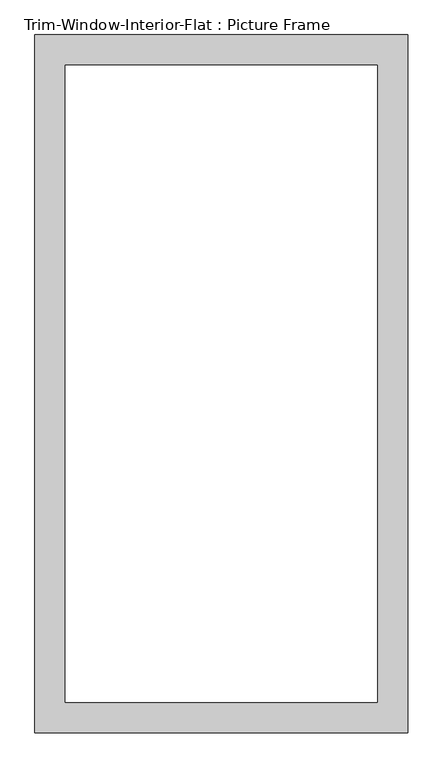
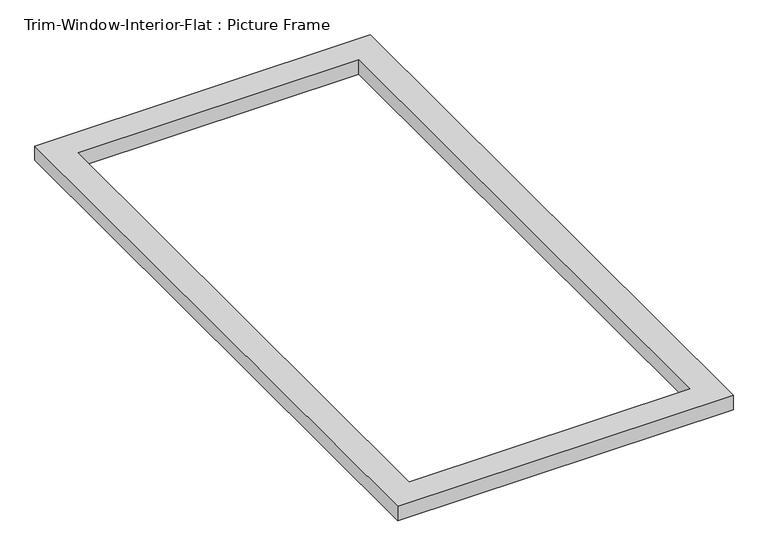
"""IFC4 building model written with IfcOpenShell, lengths in millimetres: proxy geometry, Trim-Window-Interior-Flat : Picture Frame."""

from ifc_helpers import new_model, si_unit, origin, origin_with_axes, place, context, project, spatial, polyline, outline, extrude, source, transform, mapped, element, save


def trim_window_interior_flat_picture_frame_e16bff95(model_context):
    return source(origin(), model_context, "Body", "SweptSolid", [
        extrude(outline(polyline([(349.25, 44.45), (349.25, -1263.65), (-349.25, -1263.65), (-349.25, 44.45), (349.25, 44.45)]), holes=[polyline([(292.1, -12.7), (-292.1, -12.7), (-292.1, -1206.5), (292.1, -1206.5), (292.1, -12.7)])]), origin_with_axes(), (0.0, 0.0, 1.0), 31.75),
    ])


if __name__ == "__main__":
    model = new_model("IFC4")
    model_context = context("Model", 3, world=origin())
    ifc_project = project(units=[si_unit("LENGTHUNIT", "METRE", prefix="MILLI")], contexts=[model_context])
    site = spatial("IfcSite", under=ifc_project)
    building = spatial("IfcBuilding", under=site)
    placement = place(None, origin())
    trim_window_interior_flat_picture_frame_shape = trim_window_interior_flat_picture_frame_e16bff95(model_context)
    element("IfcBuildingElementProxy", 1, Name="Trim-Window-Interior-Flat : Picture Frame", ObjectType="Trim-Window-Interior-Flat : Picture Frame", at=placement, inside=building, context=model_context, shape_type="MappedRepresentation", body=[
        mapped(trim_window_interior_flat_picture_frame_shape, transform((0.0, 0.0, 0.0), x_axis=(1.0, 0.0, 0.0), y_axis=(0.0, 1.0, 0.0), z_axis=(0.0, 0.0, 1.0))),
    ])
    save(model, "model.ifc")

# Revit data of these elements
# Type "Trim-Window-Interior-Flat : Picture Frame"
#   Trim Thickness_Picture Frame = 0' - 1 1/4"
#   Trim Width = 0' - 2 1/4"
#   Trim Thickness_with Sill = 0' - 0 3/4"
#   Sill Thickness = 0' - 1 1/4"
#   Opening Width [instance default] = 2' - 0"
#   Opening Height [instance default] = 3' - 0"
#   Default Elevation = 4' - 0"
#   Sill = no
#   Picture Frame = yes
#   Trim Material [instance default] = none
# Element 1 (IfcBuildingElementProxy, "Trim-Window-Interior-Flat : Picture Frame")
#   Opening Height = 4' - 0"
#   Trim Material = Wood - Stained
#   Materials on its faces: "Wood - Stained"
# Materials
#   "Wood - Stained": class "Wood", colour RGB 224 178 126, transparency 0, Cost = 0
